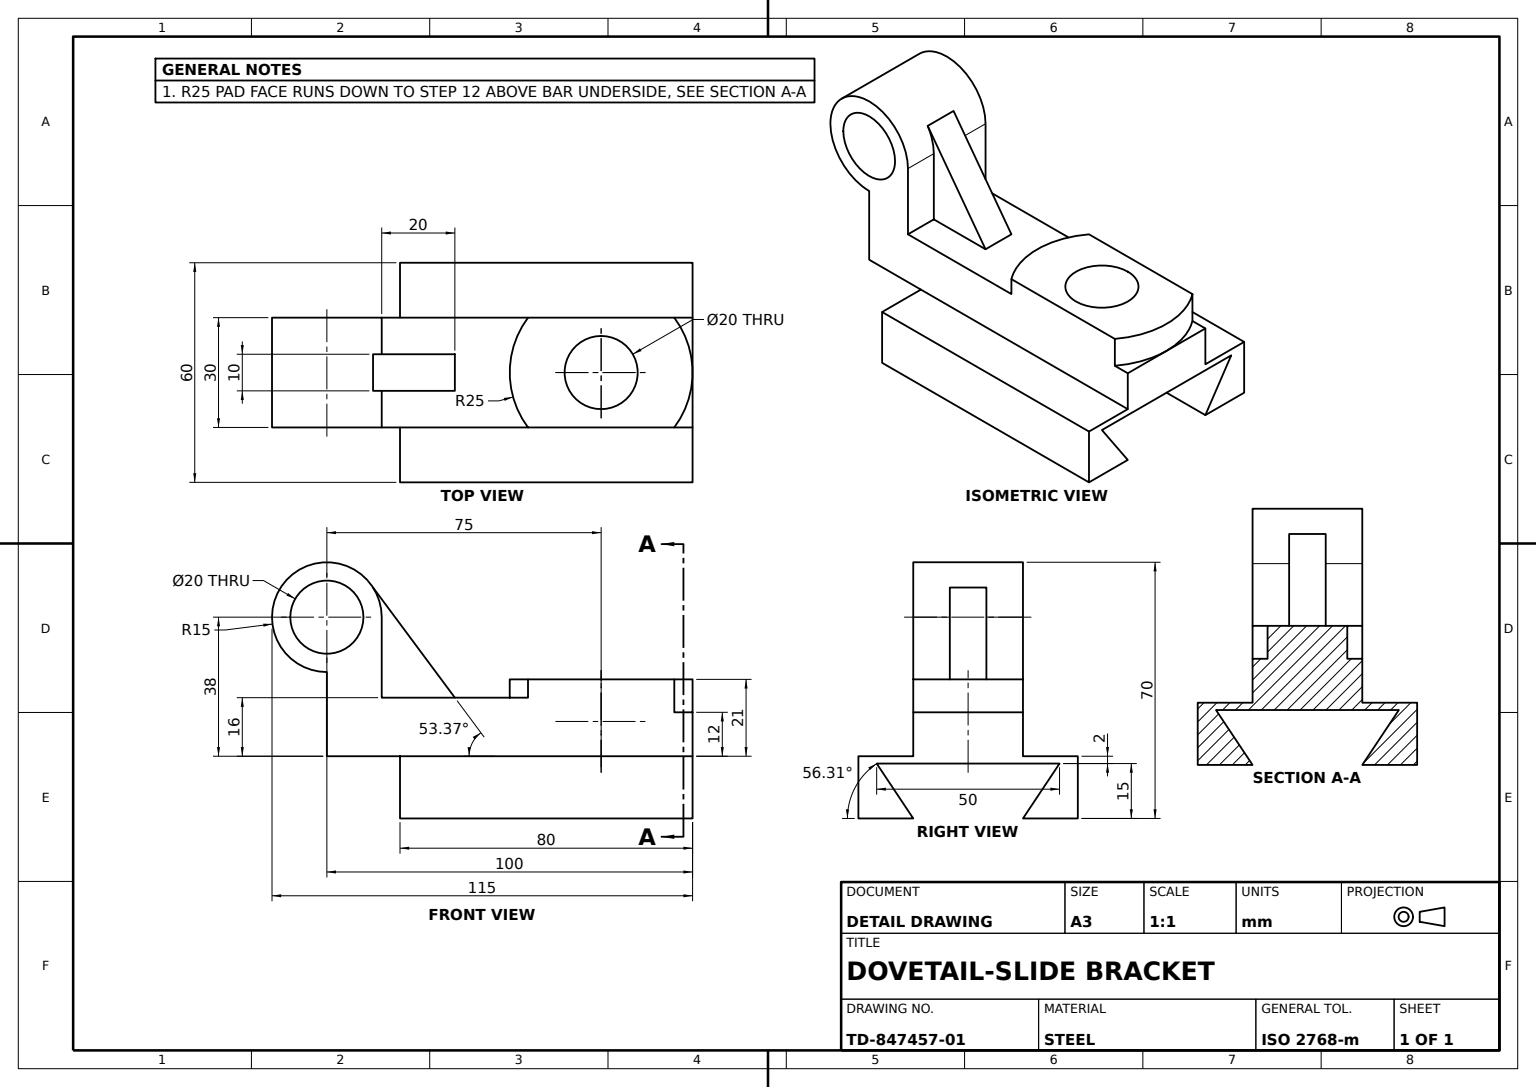
SolidWorks part; units mm, degrees
material "Plain Carbon Steel"
ref_plane "Front Plane" through (0, 0, 0) normal (0, 0, 1) x (1, 0, 0)
ref_plane "Top Plane" through (0, 0, 0) normal (0, 1, 0) x (1, 0, 0)
ref_plane "Right Plane" through (0, 0, 0) normal (1, 0, 0) x (0, 0, -1)
sketch "Base Block Profile" plane through (0, 0, 0) normal (1, 0, 0) x (0, 0, -1)
  line L0 (30, 0) -> (-30, 0)
  line L1 (-30, 0) -> (-30, -17)
  line L2 (-30, -17) -> (-15, -17)
  line L3 (-15, -17) -> (-25, -2)
  line L4 (-25, -2) -> (25, -2)
  line L5 (25, -2) -> (15, -17)
  line L6 (15, -17) -> (30, -17)
  line L7 (30, -17) -> (30, 0)
  point P4 (0, 0)
  dimension "D1" = 30
  dimension "D2" = 50
  dimension "D3" = 60
  dimension "D4" = 25
  dimension "D5" = 15
  dimension "D6" = 15
  dimension "D7" = 15
  dimension "D8" = 2
extrude "Slotted Base Block" add sketch "Base Block Profile" against normal blind 80
sketch "Pivot Pad Sketch" plane through (0, 0, 0) normal (0, 1, 0) x (1, 0, 0)
  circle A0 centre (-25, 0) radius 25
  dimension "D1" = 50
  dimension "D2" = 25
extrude "Pivot Pad Ø50" add sketch "Pivot Pad Sketch" along normal blind 21
sketch "Upper Bar Sketch" plane through (0, 0, 0) normal (1, 0, 0) x (0, 0, -1)
  line L0 (30, 0) -> (0, 0) construction
  line L1 (-15, 0) -> (15, 0)
  line L2 (-15, 0) -> (-15, 12)
  line L3 (-15, 12) -> (15, 12)
  line L4 (15, 0) -> (15, 12)
  line L7 (-25, -2) -> (25, -2) construction
  dimension "D1" = 14
  dimension "D2" = 30
  dimension "D3" = 15
extrude "Upper Bar" add sketch "Upper Bar Sketch" against normal blind 100
sketch "Through Slot Profile" plane through (0, 0, 0) normal (1, 0, 0) x (0, 0, -1)
  line L0 (30, 0) -> (15, 0) construction
  line L1 (-30, 0) -> (-15, 0)
  line L2 (-30, 0) -> (-30, 21)
  line L3 (-30, 21) -> (-15, 21)
  line L4 (-15, 0) -> (-15, 21)
  line L5 (15, 21) -> (30, 21)
  line L6 (15, 21) -> (15, 0)
  line L7 (15, 0) -> (30, 0)
  line L8 (30, 21) -> (30, 0)
  line L9 (30, -17) -> (30, 0) construction
  line L10 (25, 21) -> (-25, 21) construction
extrude "Through Slot Cut" cut sketch "Through Slot Profile" against normal blind 100
sketch "Eye Lug Reference Sketch" plane through (0, 0, 15) normal (0, 0, 1) x (1, 0, 0)
  line L1 (-100, 0) -> (-100, 51.857) construction
  line L2 (-100, 23) -> (-100, 12)
  line L3 (-100, 0) -> (-80, 0) construction
  line L10 (-85, 38) -> (-85, 16)
  line L11 (-85, 16) -> (-45, 16)
  line L12 (-45, 12) -> (-45, 21) construction
  line L13 (-100, 12) -> (-45, 12) construction
  line L14 (-100, 12) -> (-45, 12)
  line L15 (-45, 16) -> (-45, 12)
  arc A0 (-85, 38) -> (-100, 23) centre (-100, 38) ccw
  circle A1 centre (-100, 38) radius 10
  dimension "D2" = 30
  dimension "D3" = 20
  dimension "D1" = 38
  dimension "D4" = 16
sketch "Eye Lug Profile" plane through (0, 0, 0) normal (0, 0, 1) x (1, 0, 0)
  line L5 (-85, 16) -> (-85, 38)
  line L6 (-100, 23) -> (-100, 12)
  line L7 (-100, 12) -> (-45, 12)
  line L8 (-45, 12) -> (-45, 16)
  line L9 (-45, 16) -> (-85, 16)
  line L10 (-85, 16) -> (-85, 38)
  line L11 (-100, 23) -> (-100, 12)
  line L12 (-100, 12) -> (-45, 12)
  line L13 (-45, 12) -> (-45, 16)
  line L14 (-45, 16) -> (-85, 16)
  circle A1 centre (-100, 38) radius 10
  circle A2 centre (-100, 38) radius 10
  arc A3 (-85, 38) -> (-100, 23) centre (-100, 38) ccw
  arc A4 (-85, 38) -> (-100, 23) centre (-100, 38) ccw
  dimension "D1" = 0
  dimension "D2" = 0
extrude "Raised Eye Lug" add sketch "Eye Lug Profile" along normal mid plane 30
sketch "Lug Rib Sketch" plane through (0, 0, 0) normal (0, 0, 1) x (1, 0, 0)
  line L0 (-87.3735, 46.0976) -> (-65, 16)
  line L1 (-45, 16) -> (-85, 16) construction
  line L2 (-85, 16) -> (-85, 38) construction
  arc A0 (-85, 38) -> (-100, 23) centre (-100, 38) ccw construction
  dimension "D1" = 20
  dimension "D2" = 22.3735
rib "Lug Support Rib" sketch "Lug Rib Sketch" sketch "Lug Rib Sketch" thickness 10 extrusion direction parallel to sketch draft on no parameters "D1"=10
sketch "Pad Hole Sketch" plane through (0, 21, 0) normal (0, 1, 0) x (1, 0, 0)
  circle A0 centre (-25, 0) radius 10
  arc A1 (-5, -15) -> (-5, 15) centre (-25, 0) ccw construction
  dimension "D1" = 20
extrude "Pad Hole Ø20" cut sketch "Pad Hole Sketch" against normal blind 30
